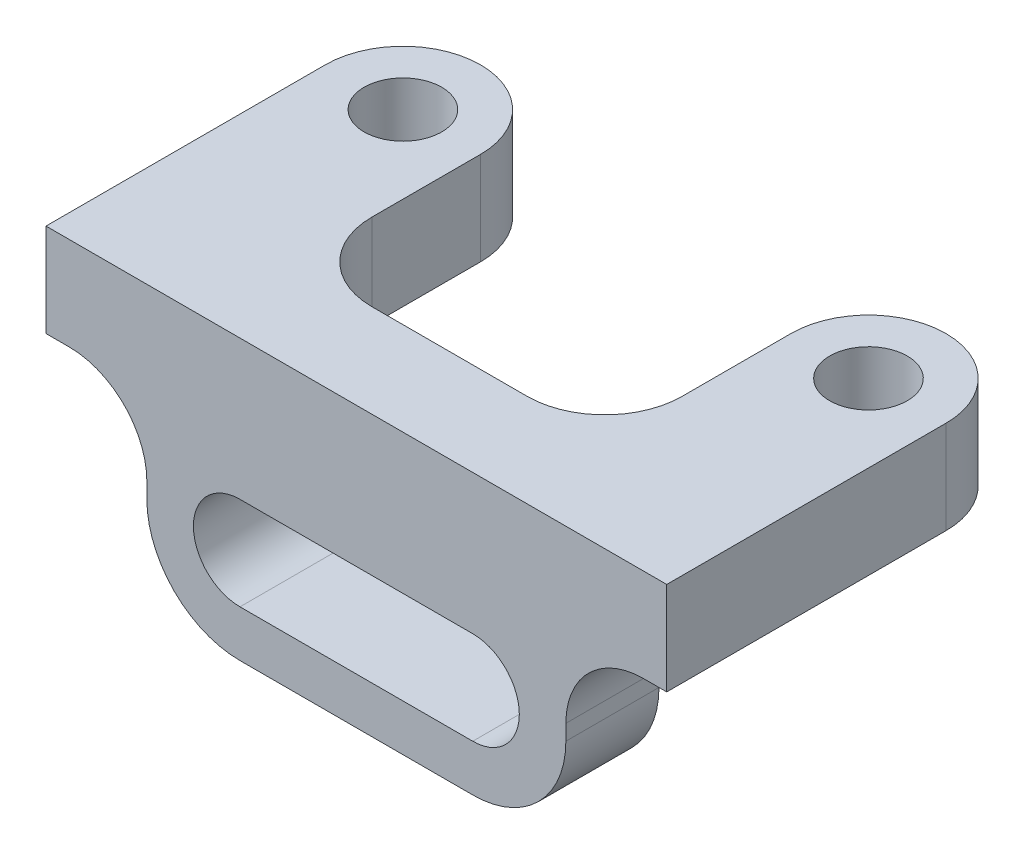
ISO-10303-21;
HEADER;
FILE_DESCRIPTION(('STEP AP214'),'2;1');
FILE_NAME('part.step','',(''),(''),'','','');
FILE_SCHEMA(('AUTOMOTIVE_DESIGN { 1 0 10303 214 1 1 1 1 }'));
ENDSEC;
DATA;
#1=APPLICATION_CONTEXT('core data for automotive mechanical design processes');
#2=APPLICATION_PROTOCOL_DEFINITION('international standard','automotive_design',2000,#1);
#3=PRODUCT_CONTEXT('',#1,'mechanical');
#4=PRODUCT('Part','Part','',(#3));
#5=PRODUCT_RELATED_PRODUCT_CATEGORY('part','',(#4));
#6=PRODUCT_DEFINITION_FORMATION('','',#4);
#7=PRODUCT_DEFINITION_CONTEXT('part definition',#1,'design');
#8=PRODUCT_DEFINITION('design','',#6,#7);
#9=PRODUCT_DEFINITION_SHAPE('','',#8);
#10=(LENGTH_UNIT() NAMED_UNIT(*) SI_UNIT(.MILLI.,.METRE.));
#11=(NAMED_UNIT(*) PLANE_ANGLE_UNIT() SI_UNIT($,.RADIAN.));
#12=(NAMED_UNIT(*) SI_UNIT($,.STERADIAN.) SOLID_ANGLE_UNIT());
#13=UNCERTAINTY_MEASURE_WITH_UNIT(LENGTH_MEASURE(1.E-05),#10,'distance_accuracy_value','');
#14=(GEOMETRIC_REPRESENTATION_CONTEXT(3) GLOBAL_UNCERTAINTY_ASSIGNED_CONTEXT((#13)) GLOBAL_UNIT_ASSIGNED_CONTEXT((#10,
#11,#12)) REPRESENTATION_CONTEXT('',''));
#15=CARTESIAN_POINT('',(0.,0.,0.));
#16=DIRECTION('',(0.,0.,1.));
#17=DIRECTION('',(1.,0.,0.));
#18=AXIS2_PLACEMENT_3D('',#15,#16,#17);
#19=CARTESIAN_POINT('',(1.5,-11.,0.));
#20=DIRECTION('',(0.,0.,1.));
#21=DIRECTION('',(1.,0.,0.));
#22=AXIS2_PLACEMENT_3D('',#19,#20,#21);
#23=PLANE('',#22);
#24=DIRECTION('',(-1.,0.,0.));
#25=VECTOR('',#24,1.);
#26=CARTESIAN_POINT('',(12.5000000000001,-15.,0.));
#27=LINE('',#26,#25);
#28=CARTESIAN_POINT('',(27.5000000000001,-15.,0.));
#29=VERTEX_POINT('',#28);
#30=CARTESIAN_POINT('',(12.5000000000001,-15.,0.));
#31=VERTEX_POINT('',#30);
#32=EDGE_CURVE('E219',#29,#31,#27,.T.);
#33=ORIENTED_EDGE('',*,*,#32,.F.);
#34=CARTESIAN_POINT('',(27.5000000000001,-12.,0.));
#35=DIRECTION('',(0.,0.,-1.));
#36=DIRECTION('',(-1.,0.,0.));
#37=AXIS2_PLACEMENT_3D('',#34,#35,#36);
#38=CIRCLE('',#37,3.);
#39=CARTESIAN_POINT('',(27.5000000000001,-9.,0.));
#40=VERTEX_POINT('',#39);
#41=EDGE_CURVE('E58',#40,#29,#38,.T.);
#42=ORIENTED_EDGE('',*,*,#41,.F.);
#43=DIRECTION('',(1.,0.,0.));
#44=VECTOR('',#43,1.);
#45=CARTESIAN_POINT('',(27.5000000000001,-9.,0.));
#46=LINE('',#45,#44);
#47=CARTESIAN_POINT('',(12.5000000000001,-9.,0.));
#48=VERTEX_POINT('',#47);
#49=EDGE_CURVE('E211',#48,#40,#46,.T.);
#50=ORIENTED_EDGE('',*,*,#49,.F.);
#51=CARTESIAN_POINT('',(12.5000000000001,-12.,0.));
#52=DIRECTION('',(0.,0.,-1.));
#53=DIRECTION('',(-1.,0.,0.));
#54=AXIS2_PLACEMENT_3D('',#51,#52,#53);
#55=CIRCLE('',#54,3.);
#56=EDGE_CURVE('E212',#31,#48,#55,.T.);
#57=ORIENTED_EDGE('',*,*,#56,.F.);
#58=EDGE_LOOP('',(#33,#42,#50,#57));
#59=FACE_BOUND('',#58,.T.);
#60=DIRECTION('',(0.,1.,0.));
#61=VECTOR('',#60,1.);
#62=CARTESIAN_POINT('',(15.,-6.,0.));
#63=LINE('',#62,#61);
#64=CARTESIAN_POINT('',(15.,-6.,0.));
#65=VERTEX_POINT('',#64);
#66=CARTESIAN_POINT('',(15.,0.,0.));
#67=VERTEX_POINT('',#66);
#68=EDGE_CURVE('E264',#65,#67,#63,.T.);
#69=ORIENTED_EDGE('',*,*,#68,.T.);
#70=DIRECTION('',(-1.,0.,0.));
#71=VECTOR('',#70,1.);
#72=CARTESIAN_POINT('',(0.,0.,0.));
#73=LINE('',#72,#71);
#74=CARTESIAN_POINT('',(25.,0.,0.));
#75=VERTEX_POINT('',#74);
#76=EDGE_CURVE('E301',#75,#67,#73,.T.);
#77=ORIENTED_EDGE('',*,*,#76,.F.);
#78=DIRECTION('',(0.,1.,0.));
#79=VECTOR('',#78,1.);
#80=CARTESIAN_POINT('',(25.,-6.,0.));
#81=LINE('',#80,#79);
#82=CARTESIAN_POINT('',(25.,-6.,0.));
#83=VERTEX_POINT('',#82);
#84=EDGE_CURVE('E282',#83,#75,#81,.T.);
#85=ORIENTED_EDGE('',*,*,#84,.F.);
#86=DIRECTION('',(1.,0.,0.));
#87=VECTOR('',#86,1.);
#88=CARTESIAN_POINT('',(25.,-6.,0.));
#89=LINE('',#88,#87);
#90=CARTESIAN_POINT('',(38.5,-6.,0.));
#91=VERTEX_POINT('',#90);
#92=EDGE_CURVE('E272',#83,#91,#89,.T.);
#93=ORIENTED_EDGE('',*,*,#92,.T.);
#94=CARTESIAN_POINT('',(38.5,-11.,0.));
#95=DIRECTION('',(0.,0.,-1.));
#96=DIRECTION('',(1.,0.,0.));
#97=AXIS2_PLACEMENT_3D('',#94,#95,#96);
#98=CIRCLE('',#97,5.);
#99=CARTESIAN_POINT('',(33.5,-11.,0.));
#100=VERTEX_POINT('',#99);
#101=EDGE_CURVE('E337',#100,#91,#98,.T.);
#102=ORIENTED_EDGE('',*,*,#101,.F.);
#103=DIRECTION('',(0.,1.,0.));
#104=VECTOR('',#103,1.);
#105=CARTESIAN_POINT('',(33.5,-12.,0.));
#106=LINE('',#105,#104);
#107=CARTESIAN_POINT('',(33.5,-12.,0.));
#108=VERTEX_POINT('',#107);
#109=EDGE_CURVE('E333',#108,#100,#106,.T.);
#110=ORIENTED_EDGE('',*,*,#109,.F.);
#111=CARTESIAN_POINT('',(27.5,-12.,0.));
#112=DIRECTION('',(0.,0.,1.));
#113=DIRECTION('',(1.,0.,0.));
#114=AXIS2_PLACEMENT_3D('',#111,#112,#113);
#115=CIRCLE('',#114,6.);
#116=CARTESIAN_POINT('',(27.5000000000001,-18.,0.));
#117=VERTEX_POINT('',#116);
#118=EDGE_CURVE('E334',#117,#108,#115,.T.);
#119=ORIENTED_EDGE('',*,*,#118,.F.);
#120=DIRECTION('',(1.,0.,0.));
#121=VECTOR('',#120,1.);
#122=CARTESIAN_POINT('',(12.5000000000001,-18.,0.));
#123=LINE('',#122,#121);
#124=CARTESIAN_POINT('',(12.5000000000001,-18.,0.));
#125=VERTEX_POINT('',#124);
#126=EDGE_CURVE('E332',#125,#117,#123,.T.);
#127=ORIENTED_EDGE('',*,*,#126,.F.);
#128=CARTESIAN_POINT('',(12.5,-12.,0.));
#129=DIRECTION('',(0.,0.,1.));
#130=DIRECTION('',(1.,0.,0.));
#131=AXIS2_PLACEMENT_3D('',#128,#129,#130);
#132=CIRCLE('',#131,6.);
#133=CARTESIAN_POINT('',(6.49999999999999,-12.,0.));
#134=VERTEX_POINT('',#133);
#135=EDGE_CURVE('E328',#134,#125,#132,.T.);
#136=ORIENTED_EDGE('',*,*,#135,.F.);
#137=DIRECTION('',(0.,-1.,0.));
#138=VECTOR('',#137,1.);
#139=CARTESIAN_POINT('',(6.5,-12.,0.));
#140=LINE('',#139,#138);
#141=CARTESIAN_POINT('',(6.5,-11.,0.));
#142=VERTEX_POINT('',#141);
#143=EDGE_CURVE('E330',#142,#134,#140,.T.);
#144=ORIENTED_EDGE('',*,*,#143,.F.);
#145=CARTESIAN_POINT('',(1.5,-11.,0.));
#146=DIRECTION('',(0.,0.,-1.));
#147=DIRECTION('',(1.,0.,0.));
#148=AXIS2_PLACEMENT_3D('',#145,#146,#147);
#149=CIRCLE('',#148,5.);
#150=CARTESIAN_POINT('',(1.5,-6.,0.));
#151=VERTEX_POINT('',#150);
#152=EDGE_CURVE('E292',#151,#142,#149,.T.);
#153=ORIENTED_EDGE('',*,*,#152,.F.);
#154=DIRECTION('',(-1.,0.,0.));
#155=VECTOR('',#154,1.);
#156=CARTESIAN_POINT('',(1.5,-6.,0.));
#157=LINE('',#156,#155);
#158=EDGE_CURVE('E11',#65,#151,#157,.T.);
#159=ORIENTED_EDGE('',*,*,#158,.F.);
#160=EDGE_LOOP('',(#69,#77,#85,#93,#102,#110,#119,#127,#136,#144,#153,#159));
#161=FACE_BOUND('',#160,.T.);
#162=ADVANCED_FACE('F44',(#59,#161),#23,.F.);
#163=CARTESIAN_POINT('',(0.,0.,6.));
#164=DIRECTION('',(1.,0.,0.));
#165=DIRECTION('',(0.,0.,-1.));
#166=AXIS2_PLACEMENT_3D('',#163,#164,#165);
#167=PLANE('',#166);
#168=DIRECTION('',(0.,0.,-1.));
#169=VECTOR('',#168,1.);
#170=CARTESIAN_POINT('',(0.,0.,6.));
#171=LINE('',#170,#169);
#172=CARTESIAN_POINT('',(0.,0.,6.));
#173=VERTEX_POINT('',#172);
#174=CARTESIAN_POINT('',(0.,0.,-12.));
#175=VERTEX_POINT('',#174);
#176=EDGE_CURVE('E324',#173,#175,#171,.T.);
#177=ORIENTED_EDGE('',*,*,#176,.T.);
#178=DIRECTION('',(0.,1.,0.));
#179=VECTOR('',#178,1.);
#180=CARTESIAN_POINT('',(0.,-6.,-12.));
#181=LINE('',#180,#179);
#182=CARTESIAN_POINT('',(0.,-6.,-12.));
#183=VERTEX_POINT('',#182);
#184=EDGE_CURVE('E252',#183,#175,#181,.T.);
#185=ORIENTED_EDGE('',*,*,#184,.F.);
#186=DIRECTION('',(0.,0.,-1.));
#187=VECTOR('',#186,1.);
#188=CARTESIAN_POINT('',(0.,-6.,6.));
#189=LINE('',#188,#187);
#190=CARTESIAN_POINT('',(0.,-6.,6.));
#191=VERTEX_POINT('',#190);
#192=EDGE_CURVE('E52',#191,#183,#189,.T.);
#193=ORIENTED_EDGE('',*,*,#192,.F.);
#194=DIRECTION('',(0.,-1.,0.));
#195=VECTOR('',#194,1.);
#196=CARTESIAN_POINT('',(0.,0.,6.));
#197=LINE('',#196,#195);
#198=EDGE_CURVE('E298',#173,#191,#197,.T.);
#199=ORIENTED_EDGE('',*,*,#198,.F.);
#200=EDGE_LOOP('',(#177,#185,#193,#199));
#201=FACE_BOUND('',#200,.T.);
#202=ADVANCED_FACE('F50',(#201),#167,.F.);
#203=CARTESIAN_POINT('',(0.,-6.,6.));
#204=DIRECTION('',(0.,1.,0.));
#205=DIRECTION('',(0.,0.,1.));
#206=AXIS2_PLACEMENT_3D('',#203,#204,#205);
#207=PLANE('',#206);
#208=CARTESIAN_POINT('',(5.,-6.,-12.));
#209=DIRECTION('',(0.,-1.,0.));
#210=DIRECTION('',(0.,0.,-1.));
#211=AXIS2_PLACEMENT_3D('',#208,#209,#210);
#212=CIRCLE('',#211,2.5);
#213=CARTESIAN_POINT('',(5.,-6.,-14.5));
#214=VERTEX_POINT('',#213);
#215=EDGE_CURVE('E234',#214,#214,#212,.T.);
#216=ORIENTED_EDGE('',*,*,#215,.F.);
#217=EDGE_LOOP('',(#216));
#218=FACE_BOUND('',#217,.T.);
#219=ORIENTED_EDGE('',*,*,#192,.T.);
#220=CARTESIAN_POINT('',(5.,-6.,-12.));
#221=DIRECTION('',(0.,1.,0.));
#222=DIRECTION('',(0.,0.,1.));
#223=AXIS2_PLACEMENT_3D('',#220,#221,#222);
#224=CIRCLE('',#223,5.);
#225=CARTESIAN_POINT('',(10.,-6.,-12.));
#226=VERTEX_POINT('',#225);
#227=EDGE_CURVE('E242',#226,#183,#224,.T.);
#228=ORIENTED_EDGE('',*,*,#227,.F.);
#229=DIRECTION('',(0.,0.,-1.));
#230=VECTOR('',#229,1.);
#231=CARTESIAN_POINT('',(10.,-6.,-12.));
#232=LINE('',#231,#230);
#233=CARTESIAN_POINT('',(10.,-6.,-5.00000000000003));
#234=VERTEX_POINT('',#233);
#235=EDGE_CURVE('E249',#234,#226,#232,.T.);
#236=ORIENTED_EDGE('',*,*,#235,.F.);
#237=CARTESIAN_POINT('',(15.,-6.,-5.));
#238=DIRECTION('',(0.,-1.,0.));
#239=DIRECTION('',(0.,0.,-1.));
#240=AXIS2_PLACEMENT_3D('',#237,#238,#239);
#241=CIRCLE('',#240,5.);
#242=EDGE_CURVE('E245',#65,#234,#241,.T.);
#243=ORIENTED_EDGE('',*,*,#242,.F.);
#244=ORIENTED_EDGE('',*,*,#158,.T.);
#245=DIRECTION('',(0.,0.,-1.));
#246=VECTOR('',#245,1.);
#247=CARTESIAN_POINT('',(1.49999999999996,-6.,6.));
#248=LINE('',#247,#246);
#249=CARTESIAN_POINT('',(1.49999999999996,-6.,6.));
#250=VERTEX_POINT('',#249);
#251=EDGE_CURVE('E366',#250,#151,#248,.T.);
#252=ORIENTED_EDGE('',*,*,#251,.F.);
#253=DIRECTION('',(1.,0.,0.));
#254=VECTOR('',#253,1.);
#255=CARTESIAN_POINT('',(0.,-6.,6.));
#256=LINE('',#255,#254);
#257=EDGE_CURVE('E305',#191,#250,#256,.T.);
#258=ORIENTED_EDGE('',*,*,#257,.F.);
#259=EDGE_LOOP('',(#219,#228,#236,#243,#244,#252,#258));
#260=FACE_BOUND('',#259,.T.);
#261=ADVANCED_FACE('F372',(#218,#260),#207,.F.);
#262=CARTESIAN_POINT('',(1.5,-11.,6.));
#263=DIRECTION('',(0.,0.,-1.));
#264=DIRECTION('',(-1.,0.,0.));
#265=AXIS2_PLACEMENT_3D('',#262,#263,#264);
#266=CYLINDRICAL_SURFACE('',#265,5.);
#267=ORIENTED_EDGE('',*,*,#152,.T.);
#268=DIRECTION('',(0.,0.,-1.));
#269=VECTOR('',#268,1.);
#270=CARTESIAN_POINT('',(6.5,-11.,6.));
#271=LINE('',#270,#269);
#272=CARTESIAN_POINT('',(6.5,-11.,6.));
#273=VERTEX_POINT('',#272);
#274=EDGE_CURVE('E364',#273,#142,#271,.T.);
#275=ORIENTED_EDGE('',*,*,#274,.F.);
#276=CARTESIAN_POINT('',(1.5,-11.,6.));
#277=DIRECTION('',(0.,0.,-1.));
#278=DIRECTION('',(1.,0.,0.));
#279=AXIS2_PLACEMENT_3D('',#276,#277,#278);
#280=CIRCLE('',#279,5.);
#281=EDGE_CURVE('E302',#250,#273,#280,.T.);
#282=ORIENTED_EDGE('',*,*,#281,.F.);
#283=ORIENTED_EDGE('',*,*,#251,.T.);
#284=EDGE_LOOP('',(#267,#275,#282,#283));
#285=FACE_BOUND('',#284,.T.);
#286=ADVANCED_FACE('F398',(#285),#266,.F.);
#287=CARTESIAN_POINT('',(6.5,-12.,6.));
#288=DIRECTION('',(1.,0.,0.));
#289=DIRECTION('',(0.,0.,-1.));
#290=AXIS2_PLACEMENT_3D('',#287,#288,#289);
#291=PLANE('',#290);
#292=ORIENTED_EDGE('',*,*,#143,.T.);
#293=DIRECTION('',(0.,0.,-1.));
#294=VECTOR('',#293,1.);
#295=CARTESIAN_POINT('',(6.49999999999999,-12.,6.));
#296=LINE('',#295,#294);
#297=CARTESIAN_POINT('',(6.49999999999999,-12.,6.));
#298=VERTEX_POINT('',#297);
#299=EDGE_CURVE('E362',#298,#134,#296,.T.);
#300=ORIENTED_EDGE('',*,*,#299,.F.);
#301=DIRECTION('',(0.,-1.,0.));
#302=VECTOR('',#301,1.);
#303=CARTESIAN_POINT('',(6.5,-12.,6.));
#304=LINE('',#303,#302);
#305=EDGE_CURVE('E307',#273,#298,#304,.T.);
#306=ORIENTED_EDGE('',*,*,#305,.F.);
#307=ORIENTED_EDGE('',*,*,#274,.T.);
#308=EDGE_LOOP('',(#292,#300,#306,#307));
#309=FACE_BOUND('',#308,.T.);
#310=ADVANCED_FACE('F397',(#309),#291,.F.);
#311=CARTESIAN_POINT('',(12.5,-12.,6.));
#312=DIRECTION('',(0.,0.,-1.));
#313=DIRECTION('',(-1.,0.,0.));
#314=AXIS2_PLACEMENT_3D('',#311,#312,#313);
#315=CYLINDRICAL_SURFACE('',#314,6.);
#316=ORIENTED_EDGE('',*,*,#135,.T.);
#317=DIRECTION('',(0.,0.,-1.));
#318=VECTOR('',#317,1.);
#319=CARTESIAN_POINT('',(12.5000000000001,-18.,6.));
#320=LINE('',#319,#318);
#321=CARTESIAN_POINT('',(12.5000000000001,-18.,6.));
#322=VERTEX_POINT('',#321);
#323=EDGE_CURVE('E359',#322,#125,#320,.T.);
#324=ORIENTED_EDGE('',*,*,#323,.F.);
#325=CARTESIAN_POINT('',(12.5,-12.,6.));
#326=DIRECTION('',(0.,0.,1.));
#327=DIRECTION('',(1.,0.,0.));
#328=AXIS2_PLACEMENT_3D('',#325,#326,#327);
#329=CIRCLE('',#328,6.);
#330=EDGE_CURVE('E310',#298,#322,#329,.T.);
#331=ORIENTED_EDGE('',*,*,#330,.F.);
#332=ORIENTED_EDGE('',*,*,#299,.T.);
#333=EDGE_LOOP('',(#316,#324,#331,#332));
#334=FACE_BOUND('',#333,.T.);
#335=ADVANCED_FACE('F460',(#334),#315,.T.);
#336=CARTESIAN_POINT('',(12.5000000000001,-18.,6.));
#337=DIRECTION('',(0.,1.,0.));
#338=DIRECTION('',(0.,0.,1.));
#339=AXIS2_PLACEMENT_3D('',#336,#337,#338);
#340=PLANE('',#339);
#341=ORIENTED_EDGE('',*,*,#126,.T.);
#342=DIRECTION('',(0.,0.,-1.));
#343=VECTOR('',#342,1.);
#344=CARTESIAN_POINT('',(27.5000000000001,-18.,6.));
#345=LINE('',#344,#343);
#346=CARTESIAN_POINT('',(27.5000000000001,-18.,6.));
#347=VERTEX_POINT('',#346);
#348=EDGE_CURVE('E358',#347,#117,#345,.T.);
#349=ORIENTED_EDGE('',*,*,#348,.F.);
#350=DIRECTION('',(1.,0.,0.));
#351=VECTOR('',#350,1.);
#352=CARTESIAN_POINT('',(12.5000000000001,-18.,6.));
#353=LINE('',#352,#351);
#354=EDGE_CURVE('E313',#322,#347,#353,.T.);
#355=ORIENTED_EDGE('',*,*,#354,.F.);
#356=ORIENTED_EDGE('',*,*,#323,.T.);
#357=EDGE_LOOP('',(#341,#349,#355,#356));
#358=FACE_BOUND('',#357,.T.);
#359=ADVANCED_FACE('F451',(#358),#340,.F.);
#360=CARTESIAN_POINT('',(27.5,-12.,6.));
#361=DIRECTION('',(0.,0.,-1.));
#362=DIRECTION('',(-1.,0.,0.));
#363=AXIS2_PLACEMENT_3D('',#360,#361,#362);
#364=CYLINDRICAL_SURFACE('',#363,6.);
#365=ORIENTED_EDGE('',*,*,#118,.T.);
#366=DIRECTION('',(0.,0.,-1.));
#367=VECTOR('',#366,1.);
#368=CARTESIAN_POINT('',(33.5,-12.,6.));
#369=LINE('',#368,#367);
#370=CARTESIAN_POINT('',(33.5,-12.,6.));
#371=VERTEX_POINT('',#370);
#372=EDGE_CURVE('E354',#371,#108,#369,.T.);
#373=ORIENTED_EDGE('',*,*,#372,.F.);
#374=CARTESIAN_POINT('',(27.5,-12.,6.));
#375=DIRECTION('',(0.,0.,1.));
#376=DIRECTION('',(1.,0.,0.));
#377=AXIS2_PLACEMENT_3D('',#374,#375,#376);
#378=CIRCLE('',#377,6.);
#379=EDGE_CURVE('E311',#347,#371,#378,.T.);
#380=ORIENTED_EDGE('',*,*,#379,.F.);
#381=ORIENTED_EDGE('',*,*,#348,.T.);
#382=EDGE_LOOP('',(#365,#373,#380,#381));
#383=FACE_BOUND('',#382,.T.);
#384=ADVANCED_FACE('F448',(#383),#364,.T.);
#385=CARTESIAN_POINT('',(33.5,-12.,6.));
#386=DIRECTION('',(-1.,0.,0.));
#387=DIRECTION('',(0.,0.,1.));
#388=AXIS2_PLACEMENT_3D('',#385,#386,#387);
#389=PLANE('',#388);
#390=ORIENTED_EDGE('',*,*,#109,.T.);
#391=DIRECTION('',(0.,0.,-1.));
#392=VECTOR('',#391,1.);
#393=CARTESIAN_POINT('',(33.5,-11.,6.));
#394=LINE('',#393,#392);
#395=CARTESIAN_POINT('',(33.5,-11.,6.));
#396=VERTEX_POINT('',#395);
#397=EDGE_CURVE('E348',#396,#100,#394,.T.);
#398=ORIENTED_EDGE('',*,*,#397,.F.);
#399=DIRECTION('',(0.,1.,0.));
#400=VECTOR('',#399,1.);
#401=CARTESIAN_POINT('',(33.5,-12.,6.));
#402=LINE('',#401,#400);
#403=EDGE_CURVE('E312',#371,#396,#402,.T.);
#404=ORIENTED_EDGE('',*,*,#403,.F.);
#405=ORIENTED_EDGE('',*,*,#372,.T.);
#406=EDGE_LOOP('',(#390,#398,#404,#405));
#407=FACE_BOUND('',#406,.T.);
#408=ADVANCED_FACE('F443',(#407),#389,.F.);
#409=CARTESIAN_POINT('',(38.5,-11.,6.));
#410=DIRECTION('',(0.,0.,-1.));
#411=DIRECTION('',(-1.,0.,0.));
#412=AXIS2_PLACEMENT_3D('',#409,#410,#411);
#413=CYLINDRICAL_SURFACE('',#412,5.);
#414=ORIENTED_EDGE('',*,*,#101,.T.);
#415=DIRECTION('',(0.,0.,-1.));
#416=VECTOR('',#415,1.);
#417=CARTESIAN_POINT('',(38.5,-6.,6.));
#418=LINE('',#417,#416);
#419=CARTESIAN_POINT('',(38.5,-6.,6.));
#420=VERTEX_POINT('',#419);
#421=EDGE_CURVE('E350',#420,#91,#418,.T.);
#422=ORIENTED_EDGE('',*,*,#421,.F.);
#423=CARTESIAN_POINT('',(38.5,-11.,6.));
#424=DIRECTION('',(0.,0.,-1.));
#425=DIRECTION('',(1.,0.,0.));
#426=AXIS2_PLACEMENT_3D('',#423,#424,#425);
#427=CIRCLE('',#426,5.);
#428=EDGE_CURVE('E320',#396,#420,#427,.T.);
#429=ORIENTED_EDGE('',*,*,#428,.F.);
#430=ORIENTED_EDGE('',*,*,#397,.T.);
#431=EDGE_LOOP('',(#414,#422,#429,#430));
#432=FACE_BOUND('',#431,.T.);
#433=ADVANCED_FACE('F442',(#432),#413,.F.);
#434=CARTESIAN_POINT('',(40.,-6.,6.));
#435=DIRECTION('',(0.,1.,0.));
#436=DIRECTION('',(0.,0.,1.));
#437=AXIS2_PLACEMENT_3D('',#434,#435,#436);
#438=PLANE('',#437);
#439=CARTESIAN_POINT('',(35.,-6.,-12.));
#440=DIRECTION('',(0.,-1.,0.));
#441=DIRECTION('',(0.,0.,-1.));
#442=AXIS2_PLACEMENT_3D('',#439,#440,#441);
#443=CIRCLE('',#442,2.5);
#444=CARTESIAN_POINT('',(35.,-6.,-14.5));
#445=VERTEX_POINT('',#444);
#446=EDGE_CURVE('E226',#445,#445,#443,.T.);
#447=ORIENTED_EDGE('',*,*,#446,.F.);
#448=EDGE_LOOP('',(#447));
#449=FACE_BOUND('',#448,.T.);
#450=ORIENTED_EDGE('',*,*,#421,.T.);
#451=ORIENTED_EDGE('',*,*,#92,.F.);
#452=CARTESIAN_POINT('',(25.,-6.,-5.));
#453=DIRECTION('',(0.,-1.,0.));
#454=DIRECTION('',(0.,0.,1.));
#455=AXIS2_PLACEMENT_3D('',#452,#453,#454);
#456=CIRCLE('',#455,5.);
#457=CARTESIAN_POINT('',(30.,-6.,-5.00000000000004));
#458=VERTEX_POINT('',#457);
#459=EDGE_CURVE('E269',#458,#83,#456,.T.);
#460=ORIENTED_EDGE('',*,*,#459,.F.);
#461=DIRECTION('',(0.,0.,1.));
#462=VECTOR('',#461,1.);
#463=CARTESIAN_POINT('',(30.,-6.,-12.));
#464=LINE('',#463,#462);
#465=CARTESIAN_POINT('',(30.,-6.,-12.));
#466=VERTEX_POINT('',#465);
#467=EDGE_CURVE('E276',#466,#458,#464,.T.);
#468=ORIENTED_EDGE('',*,*,#467,.F.);
#469=CARTESIAN_POINT('',(35.,-6.,-12.));
#470=DIRECTION('',(0.,1.,0.));
#471=DIRECTION('',(0.,0.,1.));
#472=AXIS2_PLACEMENT_3D('',#469,#470,#471);
#473=CIRCLE('',#472,5.);
#474=CARTESIAN_POINT('',(40.,-6.,-12.));
#475=VERTEX_POINT('',#474);
#476=EDGE_CURVE('E277',#475,#466,#473,.T.);
#477=ORIENTED_EDGE('',*,*,#476,.F.);
#478=DIRECTION('',(0.,0.,-1.));
#479=VECTOR('',#478,1.);
#480=CARTESIAN_POINT('',(40.,-6.,6.));
#481=LINE('',#480,#479);
#482=CARTESIAN_POINT('',(40.,-6.,6.));
#483=VERTEX_POINT('',#482);
#484=EDGE_CURVE('E342',#483,#475,#481,.T.);
#485=ORIENTED_EDGE('',*,*,#484,.F.);
#486=DIRECTION('',(1.,0.,0.));
#487=VECTOR('',#486,1.);
#488=CARTESIAN_POINT('',(40.,-6.,6.));
#489=LINE('',#488,#487);
#490=EDGE_CURVE('E317',#420,#483,#489,.T.);
#491=ORIENTED_EDGE('',*,*,#490,.F.);
#492=EDGE_LOOP('',(#450,#451,#460,#468,#477,#485,#491));
#493=FACE_BOUND('',#492,.T.);
#494=ADVANCED_FACE('F440',(#449,#493),#438,.F.);
#495=CARTESIAN_POINT('',(40.,0.,6.));
#496=DIRECTION('',(-1.,0.,0.));
#497=DIRECTION('',(0.,0.,1.));
#498=AXIS2_PLACEMENT_3D('',#495,#496,#497);
#499=PLANE('',#498);
#500=ORIENTED_EDGE('',*,*,#484,.T.);
#501=DIRECTION('',(0.,1.,0.));
#502=VECTOR('',#501,1.);
#503=CARTESIAN_POINT('',(40.,-6.,-12.));
#504=LINE('',#503,#502);
#505=CARTESIAN_POINT('',(40.,0.,-12.));
#506=VERTEX_POINT('',#505);
#507=EDGE_CURVE('E294',#475,#506,#504,.T.);
#508=ORIENTED_EDGE('',*,*,#507,.T.);
#509=DIRECTION('',(0.,0.,-1.));
#510=VECTOR('',#509,1.);
#511=CARTESIAN_POINT('',(40.,0.,6.));
#512=LINE('',#511,#510);
#513=CARTESIAN_POINT('',(40.,0.,6.));
#514=VERTEX_POINT('',#513);
#515=EDGE_CURVE('E341',#514,#506,#512,.T.);
#516=ORIENTED_EDGE('',*,*,#515,.F.);
#517=DIRECTION('',(0.,1.,0.));
#518=VECTOR('',#517,1.);
#519=CARTESIAN_POINT('',(40.,0.,6.));
#520=LINE('',#519,#518);
#521=EDGE_CURVE('E321',#483,#514,#520,.T.);
#522=ORIENTED_EDGE('',*,*,#521,.F.);
#523=EDGE_LOOP('',(#500,#508,#516,#522));
#524=FACE_BOUND('',#523,.T.);
#525=ADVANCED_FACE('F433',(#524),#499,.F.);
#526=CARTESIAN_POINT('',(0.,0.,6.));
#527=DIRECTION('',(0.,-1.,0.));
#528=DIRECTION('',(0.,0.,-1.));
#529=AXIS2_PLACEMENT_3D('',#526,#527,#528);
#530=PLANE('',#529);
#531=CARTESIAN_POINT('',(5.,0.,-12.));
#532=DIRECTION('',(0.,-1.,0.));
#533=DIRECTION('',(0.,0.,-1.));
#534=AXIS2_PLACEMENT_3D('',#531,#532,#533);
#535=CIRCLE('',#534,2.5);
#536=CARTESIAN_POINT('',(5.,0.,-14.5));
#537=VERTEX_POINT('',#536);
#538=EDGE_CURVE('E230',#537,#537,#535,.T.);
#539=ORIENTED_EDGE('',*,*,#538,.T.);
#540=EDGE_LOOP('',(#539));
#541=FACE_BOUND('',#540,.T.);
#542=CARTESIAN_POINT('',(35.,0.,-12.));
#543=DIRECTION('',(0.,-1.,0.));
#544=DIRECTION('',(0.,0.,-1.));
#545=AXIS2_PLACEMENT_3D('',#542,#543,#544);
#546=CIRCLE('',#545,2.5);
#547=CARTESIAN_POINT('',(35.,0.,-14.5));
#548=VERTEX_POINT('',#547);
#549=EDGE_CURVE('E240',#548,#548,#546,.T.);
#550=ORIENTED_EDGE('',*,*,#549,.T.);
#551=EDGE_LOOP('',(#550));
#552=FACE_BOUND('',#551,.T.);
#553=ORIENTED_EDGE('',*,*,#515,.T.);
#554=CARTESIAN_POINT('',(35.,0.,-12.));
#555=DIRECTION('',(0.,1.,0.));
#556=DIRECTION('',(0.,0.,1.));
#557=AXIS2_PLACEMENT_3D('',#554,#555,#556);
#558=CIRCLE('',#557,5.);
#559=CARTESIAN_POINT('',(30.,0.,-12.));
#560=VERTEX_POINT('',#559);
#561=EDGE_CURVE('E283',#506,#560,#558,.T.);
#562=ORIENTED_EDGE('',*,*,#561,.T.);
#563=DIRECTION('',(0.,0.,1.));
#564=VECTOR('',#563,1.);
#565=CARTESIAN_POINT('',(30.,0.,-12.));
#566=LINE('',#565,#564);
#567=CARTESIAN_POINT('',(30.,0.,-5.00000000000004));
#568=VERTEX_POINT('',#567);
#569=EDGE_CURVE('E273',#560,#568,#566,.T.);
#570=ORIENTED_EDGE('',*,*,#569,.T.);
#571=CARTESIAN_POINT('',(25.,0.,-5.));
#572=DIRECTION('',(0.,-1.,0.));
#573=DIRECTION('',(0.,0.,1.));
#574=AXIS2_PLACEMENT_3D('',#571,#572,#573);
#575=CIRCLE('',#574,5.);
#576=EDGE_CURVE('E265',#568,#75,#575,.T.);
#577=ORIENTED_EDGE('',*,*,#576,.T.);
#578=ORIENTED_EDGE('',*,*,#76,.T.);
#579=CARTESIAN_POINT('',(15.,0.,-5.));
#580=DIRECTION('',(0.,-1.,0.));
#581=DIRECTION('',(0.,0.,-1.));
#582=AXIS2_PLACEMENT_3D('',#579,#580,#581);
#583=CIRCLE('',#582,5.);
#584=CARTESIAN_POINT('',(10.,0.,-5.00000000000003));
#585=VERTEX_POINT('',#584);
#586=EDGE_CURVE('E254',#67,#585,#583,.T.);
#587=ORIENTED_EDGE('',*,*,#586,.T.);
#588=DIRECTION('',(0.,0.,-1.));
#589=VECTOR('',#588,1.);
#590=CARTESIAN_POINT('',(10.,0.,-12.));
#591=LINE('',#590,#589);
#592=CARTESIAN_POINT('',(10.,0.,-12.));
#593=VERTEX_POINT('',#592);
#594=EDGE_CURVE('E248',#585,#593,#591,.T.);
#595=ORIENTED_EDGE('',*,*,#594,.T.);
#596=CARTESIAN_POINT('',(5.,0.,-12.));
#597=DIRECTION('',(0.,1.,0.));
#598=DIRECTION('',(0.,0.,1.));
#599=AXIS2_PLACEMENT_3D('',#596,#597,#598);
#600=CIRCLE('',#599,5.);
#601=EDGE_CURVE('E231',#593,#175,#600,.T.);
#602=ORIENTED_EDGE('',*,*,#601,.T.);
#603=ORIENTED_EDGE('',*,*,#176,.F.);
#604=DIRECTION('',(-1.,0.,0.));
#605=VECTOR('',#604,1.);
#606=CARTESIAN_POINT('',(0.,0.,6.));
#607=LINE('',#606,#605);
#608=EDGE_CURVE('E323',#514,#173,#607,.T.);
#609=ORIENTED_EDGE('',*,*,#608,.F.);
#610=EDGE_LOOP('',(#553,#562,#570,#577,#578,#587,#595,#602,#603,#609));
#611=FACE_BOUND('',#610,.T.);
#612=ADVANCED_FACE('F409',(#541,#552,#611),#530,.F.);
#613=CARTESIAN_POINT('',(1.5,-11.,6.));
#614=DIRECTION('',(0.,0.,1.));
#615=DIRECTION('',(1.,0.,0.));
#616=AXIS2_PLACEMENT_3D('',#613,#614,#615);
#617=PLANE('',#616);
#618=CARTESIAN_POINT('',(27.5000000000001,-12.,6.));
#619=DIRECTION('',(0.,0.,-1.));
#620=DIRECTION('',(-1.,0.,0.));
#621=AXIS2_PLACEMENT_3D('',#618,#619,#620);
#622=CIRCLE('',#621,3.);
#623=CARTESIAN_POINT('',(27.5000000000001,-9.,6.));
#624=VERTEX_POINT('',#623);
#625=CARTESIAN_POINT('',(27.5000000000001,-15.,6.));
#626=VERTEX_POINT('',#625);
#627=EDGE_CURVE('E192',#624,#626,#622,.T.);
#628=ORIENTED_EDGE('',*,*,#627,.T.);
#629=DIRECTION('',(-1.,0.,0.));
#630=VECTOR('',#629,1.);
#631=CARTESIAN_POINT('',(12.5000000000001,-15.,6.));
#632=LINE('',#631,#630);
#633=CARTESIAN_POINT('',(12.5000000000001,-15.,6.));
#634=VERTEX_POINT('',#633);
#635=EDGE_CURVE('E204',#626,#634,#632,.T.);
#636=ORIENTED_EDGE('',*,*,#635,.T.);
#637=CARTESIAN_POINT('',(12.5000000000001,-12.,6.));
#638=DIRECTION('',(0.,0.,-1.));
#639=DIRECTION('',(-1.,0.,0.));
#640=AXIS2_PLACEMENT_3D('',#637,#638,#639);
#641=CIRCLE('',#640,3.);
#642=CARTESIAN_POINT('',(12.5000000000001,-9.,6.));
#643=VERTEX_POINT('',#642);
#644=EDGE_CURVE('E66',#634,#643,#641,.T.);
#645=ORIENTED_EDGE('',*,*,#644,.T.);
#646=DIRECTION('',(1.,0.,0.));
#647=VECTOR('',#646,1.);
#648=CARTESIAN_POINT('',(27.5000000000001,-9.,6.));
#649=LINE('',#648,#647);
#650=EDGE_CURVE('E203',#643,#624,#649,.T.);
#651=ORIENTED_EDGE('',*,*,#650,.T.);
#652=EDGE_LOOP('',(#628,#636,#645,#651));
#653=FACE_BOUND('',#652,.T.);
#654=ORIENTED_EDGE('',*,*,#198,.T.);
#655=ORIENTED_EDGE('',*,*,#257,.T.);
#656=ORIENTED_EDGE('',*,*,#281,.T.);
#657=ORIENTED_EDGE('',*,*,#305,.T.);
#658=ORIENTED_EDGE('',*,*,#330,.T.);
#659=ORIENTED_EDGE('',*,*,#354,.T.);
#660=ORIENTED_EDGE('',*,*,#379,.T.);
#661=ORIENTED_EDGE('',*,*,#403,.T.);
#662=ORIENTED_EDGE('',*,*,#428,.T.);
#663=ORIENTED_EDGE('',*,*,#490,.T.);
#664=ORIENTED_EDGE('',*,*,#521,.T.);
#665=ORIENTED_EDGE('',*,*,#608,.T.);
#666=EDGE_LOOP('',(#654,#655,#656,#657,#658,#659,#660,#661,#662,#663,#664,#665));
#667=FACE_BOUND('',#666,.T.);
#668=ADVANCED_FACE('F208',(#653,#667),#617,.T.);
#669=CARTESIAN_POINT('',(25.,-6.,-5.));
#670=DIRECTION('',(0.,1.,0.));
#671=DIRECTION('',(0.,0.,1.));
#672=AXIS2_PLACEMENT_3D('',#669,#670,#671);
#673=CYLINDRICAL_SURFACE('',#672,5.);
#674=ORIENTED_EDGE('',*,*,#576,.F.);
#675=DIRECTION('',(0.,1.,0.));
#676=VECTOR('',#675,1.);
#677=CARTESIAN_POINT('',(30.,-6.,-5.00000000000004));
#678=LINE('',#677,#676);
#679=EDGE_CURVE('E289',#458,#568,#678,.T.);
#680=ORIENTED_EDGE('',*,*,#679,.F.);
#681=ORIENTED_EDGE('',*,*,#459,.T.);
#682=ORIENTED_EDGE('',*,*,#84,.T.);
#683=EDGE_LOOP('',(#674,#680,#681,#682));
#684=FACE_BOUND('',#683,.T.);
#685=ADVANCED_FACE('F535',(#684),#673,.F.);
#686=CARTESIAN_POINT('',(30.,-6.,-12.));
#687=DIRECTION('',(-1.,0.,0.));
#688=DIRECTION('',(0.,0.,1.));
#689=AXIS2_PLACEMENT_3D('',#686,#687,#688);
#690=PLANE('',#689);
#691=ORIENTED_EDGE('',*,*,#569,.F.);
#692=DIRECTION('',(0.,1.,0.));
#693=VECTOR('',#692,1.);
#694=CARTESIAN_POINT('',(30.,-6.,-12.));
#695=LINE('',#694,#693);
#696=EDGE_CURVE('E295',#466,#560,#695,.T.);
#697=ORIENTED_EDGE('',*,*,#696,.F.);
#698=ORIENTED_EDGE('',*,*,#467,.T.);
#699=ORIENTED_EDGE('',*,*,#679,.T.);
#700=EDGE_LOOP('',(#691,#697,#698,#699));
#701=FACE_BOUND('',#700,.T.);
#702=ADVANCED_FACE('F689',(#701),#690,.T.);
#703=CARTESIAN_POINT('',(35.,-6.,-12.));
#704=DIRECTION('',(0.,1.,0.));
#705=DIRECTION('',(0.,0.,1.));
#706=AXIS2_PLACEMENT_3D('',#703,#704,#705);
#707=CYLINDRICAL_SURFACE('',#706,5.);
#708=ORIENTED_EDGE('',*,*,#561,.F.);
#709=ORIENTED_EDGE('',*,*,#507,.F.);
#710=ORIENTED_EDGE('',*,*,#476,.T.);
#711=ORIENTED_EDGE('',*,*,#696,.T.);
#712=EDGE_LOOP('',(#708,#709,#710,#711));
#713=FACE_BOUND('',#712,.T.);
#714=ADVANCED_FACE('F700',(#713),#707,.T.);
#715=CARTESIAN_POINT('',(5.,-6.,-12.));
#716=DIRECTION('',(0.,1.,0.));
#717=DIRECTION('',(0.,0.,1.));
#718=AXIS2_PLACEMENT_3D('',#715,#716,#717);
#719=CYLINDRICAL_SURFACE('',#718,5.);
#720=ORIENTED_EDGE('',*,*,#601,.F.);
#721=DIRECTION('',(0.,1.,0.));
#722=VECTOR('',#721,1.);
#723=CARTESIAN_POINT('',(10.,-6.,-12.));
#724=LINE('',#723,#722);
#725=EDGE_CURVE('E257',#226,#593,#724,.T.);
#726=ORIENTED_EDGE('',*,*,#725,.F.);
#727=ORIENTED_EDGE('',*,*,#227,.T.);
#728=ORIENTED_EDGE('',*,*,#184,.T.);
#729=EDGE_LOOP('',(#720,#726,#727,#728));
#730=FACE_BOUND('',#729,.T.);
#731=ADVANCED_FACE('F385',(#730),#719,.T.);
#732=CARTESIAN_POINT('',(10.,-6.,-12.));
#733=DIRECTION('',(1.,0.,0.));
#734=DIRECTION('',(0.,0.,-1.));
#735=AXIS2_PLACEMENT_3D('',#732,#733,#734);
#736=PLANE('',#735);
#737=ORIENTED_EDGE('',*,*,#594,.F.);
#738=DIRECTION('',(0.,1.,0.));
#739=VECTOR('',#738,1.);
#740=CARTESIAN_POINT('',(10.,-6.,-5.00000000000003));
#741=LINE('',#740,#739);
#742=EDGE_CURVE('E263',#234,#585,#741,.T.);
#743=ORIENTED_EDGE('',*,*,#742,.F.);
#744=ORIENTED_EDGE('',*,*,#235,.T.);
#745=ORIENTED_EDGE('',*,*,#725,.T.);
#746=EDGE_LOOP('',(#737,#743,#744,#745));
#747=FACE_BOUND('',#746,.T.);
#748=ADVANCED_FACE('F384',(#747),#736,.T.);
#749=CARTESIAN_POINT('',(15.,-6.,-5.));
#750=DIRECTION('',(0.,1.,0.));
#751=DIRECTION('',(0.,0.,1.));
#752=AXIS2_PLACEMENT_3D('',#749,#750,#751);
#753=CYLINDRICAL_SURFACE('',#752,5.);
#754=ORIENTED_EDGE('',*,*,#586,.F.);
#755=ORIENTED_EDGE('',*,*,#68,.F.);
#756=ORIENTED_EDGE('',*,*,#242,.T.);
#757=ORIENTED_EDGE('',*,*,#742,.T.);
#758=EDGE_LOOP('',(#754,#755,#756,#757));
#759=FACE_BOUND('',#758,.T.);
#760=ADVANCED_FACE('F408',(#759),#753,.F.);
#761=CARTESIAN_POINT('',(35.,0.,-12.));
#762=DIRECTION('',(0.,-1.,0.));
#763=DIRECTION('',(0.,0.,-1.));
#764=AXIS2_PLACEMENT_3D('',#761,#762,#763);
#765=CYLINDRICAL_SURFACE('',#764,2.5);
#766=ORIENTED_EDGE('',*,*,#549,.F.);
#767=EDGE_LOOP('',(#766));
#768=FACE_BOUND('',#767,.T.);
#769=ORIENTED_EDGE('',*,*,#446,.T.);
#770=EDGE_LOOP('',(#769));
#771=FACE_BOUND('',#770,.T.);
#772=ADVANCED_FACE('F413',(#768,#771),#765,.F.);
#773=CARTESIAN_POINT('',(5.,0.,-12.));
#774=DIRECTION('',(0.,-1.,0.));
#775=DIRECTION('',(0.,0.,-1.));
#776=AXIS2_PLACEMENT_3D('',#773,#774,#775);
#777=CYLINDRICAL_SURFACE('',#776,2.5);
#778=ORIENTED_EDGE('',*,*,#538,.F.);
#779=EDGE_LOOP('',(#778));
#780=FACE_BOUND('',#779,.T.);
#781=ORIENTED_EDGE('',*,*,#215,.T.);
#782=EDGE_LOOP('',(#781));
#783=FACE_BOUND('',#782,.T.);
#784=ADVANCED_FACE('F417',(#780,#783),#777,.F.);
#785=CARTESIAN_POINT('',(27.5000000000001,-12.,6.));
#786=DIRECTION('',(0.,0.,-1.));
#787=DIRECTION('',(-1.,0.,0.));
#788=AXIS2_PLACEMENT_3D('',#785,#786,#787);
#789=CYLINDRICAL_SURFACE('',#788,3.);
#790=ORIENTED_EDGE('',*,*,#41,.T.);
#791=DIRECTION('',(0.,0.,-1.));
#792=VECTOR('',#791,1.);
#793=CARTESIAN_POINT('',(27.5000000000001,-15.,6.));
#794=LINE('',#793,#792);
#795=EDGE_CURVE('E193',#626,#29,#794,.T.);
#796=ORIENTED_EDGE('',*,*,#795,.F.);
#797=ORIENTED_EDGE('',*,*,#627,.F.);
#798=DIRECTION('',(0.,0.,-1.));
#799=VECTOR('',#798,1.);
#800=CARTESIAN_POINT('',(27.5000000000001,-9.,6.));
#801=LINE('',#800,#799);
#802=EDGE_CURVE('E221',#624,#40,#801,.T.);
#803=ORIENTED_EDGE('',*,*,#802,.T.);
#804=EDGE_LOOP('',(#790,#796,#797,#803));
#805=FACE_BOUND('',#804,.T.);
#806=ADVANCED_FACE('F191',(#805),#789,.F.);
#807=CARTESIAN_POINT('',(27.5000000000001,-9.,6.));
#808=DIRECTION('',(0.,1.,0.));
#809=DIRECTION('',(0.,0.,1.));
#810=AXIS2_PLACEMENT_3D('',#807,#808,#809);
#811=PLANE('',#810);
#812=ORIENTED_EDGE('',*,*,#49,.T.);
#813=ORIENTED_EDGE('',*,*,#802,.F.);
#814=ORIENTED_EDGE('',*,*,#650,.F.);
#815=DIRECTION('',(0.,0.,-1.));
#816=VECTOR('',#815,1.);
#817=CARTESIAN_POINT('',(12.5000000000001,-9.,6.));
#818=LINE('',#817,#816);
#819=EDGE_CURVE('E227',#643,#48,#818,.T.);
#820=ORIENTED_EDGE('',*,*,#819,.T.);
#821=EDGE_LOOP('',(#812,#813,#814,#820));
#822=FACE_BOUND('',#821,.T.);
#823=ADVANCED_FACE('F476',(#822),#811,.F.);
#824=CARTESIAN_POINT('',(12.5000000000001,-12.,6.));
#825=DIRECTION('',(0.,0.,-1.));
#826=DIRECTION('',(-1.,0.,0.));
#827=AXIS2_PLACEMENT_3D('',#824,#825,#826);
#828=CYLINDRICAL_SURFACE('',#827,3.);
#829=ORIENTED_EDGE('',*,*,#56,.T.);
#830=ORIENTED_EDGE('',*,*,#819,.F.);
#831=ORIENTED_EDGE('',*,*,#644,.F.);
#832=DIRECTION('',(0.,0.,-1.));
#833=VECTOR('',#832,1.);
#834=CARTESIAN_POINT('',(12.5000000000001,-15.,6.));
#835=LINE('',#834,#833);
#836=EDGE_CURVE('E199',#634,#31,#835,.T.);
#837=ORIENTED_EDGE('',*,*,#836,.T.);
#838=EDGE_LOOP('',(#829,#830,#831,#837));
#839=FACE_BOUND('',#838,.T.);
#840=ADVANCED_FACE('F482',(#839),#828,.F.);
#841=CARTESIAN_POINT('',(12.5000000000001,-15.,6.));
#842=DIRECTION('',(0.,-1.,0.));
#843=DIRECTION('',(0.,0.,-1.));
#844=AXIS2_PLACEMENT_3D('',#841,#842,#843);
#845=PLANE('',#844);
#846=ORIENTED_EDGE('',*,*,#32,.T.);
#847=ORIENTED_EDGE('',*,*,#836,.F.);
#848=ORIENTED_EDGE('',*,*,#635,.F.);
#849=ORIENTED_EDGE('',*,*,#795,.T.);
#850=EDGE_LOOP('',(#846,#847,#848,#849));
#851=FACE_BOUND('',#850,.T.);
#852=ADVANCED_FACE('F202',(#851),#845,.F.);
#853=CLOSED_SHELL('',(#162,#202,#261,#286,#310,#335,#359,#384,#408,#433,#494,#525,#612,#668,
#685,#702,#714,#731,#748,#760,#772,#784,#806,#823,#840,#852));
#854=MANIFOLD_SOLID_BREP('B2',#853);
#855=ADVANCED_BREP_SHAPE_REPRESENTATION('',(#18,#854),#14);
#856=SHAPE_DEFINITION_REPRESENTATION(#9,#855);
ENDSEC;
END-ISO-10303-21;
